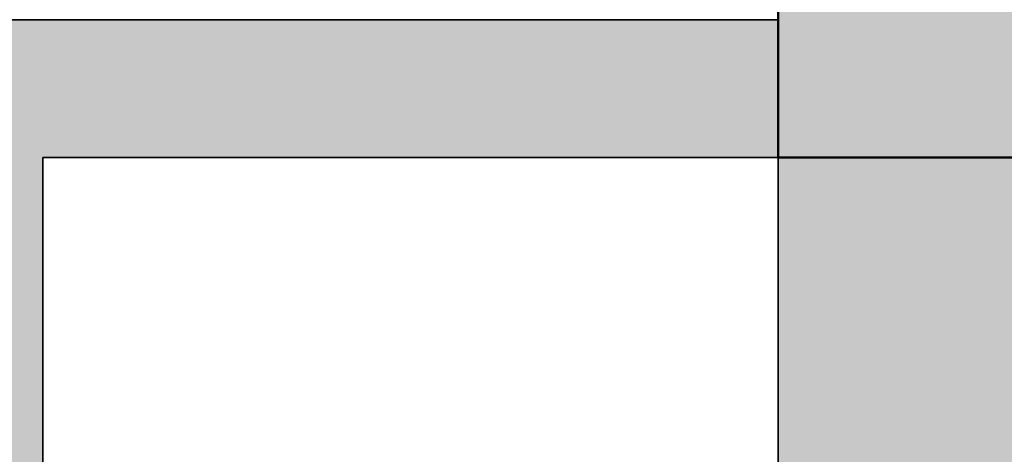
# Model space of a CAD drawing. Units: inches. Extents: x 1998 to 2588, y 1139 to 1977.
# Tile 59 of 134: x 2063 to 2095, y 1746 to 1760. Entities that reach past the tile are written whole.
import ezdxf

# ---------------------------------------------------------------- set-up
doc = ezdxf.new("R2010")
doc.units = ezdxf.units.IN
for name, color, linetype, lineweight in [('A-COLS-PATT', 250, 'Continuous', 13), ('A-WALL-PATT', 252, 'Continuous', 13), ('COLUMN', 10, 'Continuous', 50), ('WALL', 200, 'Continuous', 35)]:
    doc.layers.add(name, color=color, linetype=linetype, lineweight=lineweight)

msp = doc.modelspace()

# ---------------------------------------------------------------- hatches: boundary and pattern name
at = {"layer": 'A-COLS-PATT'}
h = msp.add_hatch(color=256, dxfattribs=at)
h.dxf.hatch_style = 1
h.paths.add_polyline_path([(2099.4125, 1888.7324), (2087.9729, 1888.7324), (2087.9729, 1868.3278), (2099.4125, 1868.3278)])
h.paths.add_polyline_path([(2234.4125, 1888.7324), (2222.9729, 1888.7324), (2222.9729, 1868.3278), (2234.4125, 1868.3278)])
h.paths.add_polyline_path([(2341.4729, 1886.637), (2330.0332, 1886.637), (2330.0332, 1866.2324), (2341.4729, 1866.2324)])
h.paths.add_polyline_path([(2507.8006, 1882.7324), (2487.396, 1882.7324), (2487.396, 1871.2927), (2507.8006, 1871.2927)])
h.paths.add_polyline_path([(2510.9729, 1766.672), (2490.5682, 1766.672), (2490.5682, 1755.2324), (2510.9729, 1755.2324)])
h.paths.add_polyline_path([(2345.9729, 1759.7324), (2334.5332, 1759.7324), (2334.5332, 1739.3278), (2345.9729, 1739.3278)])
h.paths.add_polyline_path([(2234.4125, 1774.3318), (2222.9729, 1774.3318), (2222.9729, 1753.9272), (2234.4125, 1753.9272)])
h.paths.add_polyline_path([(2099.4125, 1775.637), (2087.9729, 1775.637), (2087.9729, 1755.2324), (2099.4125, 1755.2324)])
h.paths.add_polyline_path([(2098.0956, 1593.7241), (2077.691, 1593.7241), (2077.691, 1582.2845), (2098.0956, 1582.2845)])
h.paths.add_polyline_path([(2227.4729, 1604.637), (2216.0332, 1604.637), (2216.0332, 1584.2324), (2227.4729, 1584.2324)])
h.paths.add_polyline_path([(2345.9729, 1647.5211), (2334.5332, 1647.5211), (2334.5332, 1627.1165), (2345.9729, 1627.1165)])
h.paths.add_polyline_path([(2522.3775, 1641.2324), (2501.9729, 1641.2324), (2501.9729, 1629.7927), (2522.3775, 1629.7927)])
h.paths.add_polyline_path([(2522.3775, 1480.7324), (2501.9729, 1480.7324), (2501.9729, 1469.2927), (2522.3775, 1469.2927)])
h.paths.add_polyline_path([(2345.9729, 1488.5616), (2334.5332, 1488.5616), (2334.5332, 1468.1569), (2345.9729, 1468.1569)])
h.paths.add_polyline_path([(2234.4125, 1486.137), (2227.4729, 1486.137), (2227.4729, 1465.7324), (2234.4125, 1465.7324)])
h.paths.add_polyline_path([(2227.4729, 1486.137), (2222.9729, 1486.137), (2222.9729, 1465.7324), (2227.4729, 1465.7324)])
h.paths.add_polyline_path([(2108.3775, 1470.2324), (2087.9729, 1470.2324), (2087.9729, 1458.7927), (2108.3775, 1458.7927)])
h.paths.add_polyline_path([(2096.9729, 1365.5012), (2087.9729, 1365.5012), (2087.9729, 1345.0966), (2096.9729, 1345.0966)])
h.paths.add_polyline_path([(2087.9729, 1365.5012), (2085.5332, 1365.5012), (2085.5332, 1345.0966), (2087.9729, 1345.0966)])
h.paths.add_polyline_path([(2234.4125, 1285.137), (2222.9729, 1285.137), (2222.9729, 1264.7324), (2234.4125, 1264.7324)])
h.paths.add_polyline_path([(2345.9729, 1285.137), (2334.5332, 1285.137), (2334.5332, 1264.7324), (2345.9729, 1264.7324)])
h.paths.add_polyline_path([(2503.1458, 1240.172), (2482.7412, 1240.172), (2482.7412, 1228.7324), (2503.1458, 1228.7324)])
h.paths.add_polyline_path([(2510.9729, 1369.172), (2490.5682, 1369.172), (2490.5682, 1357.7324), (2510.9729, 1357.7324)])
at = {"layer": 'A-WALL-PATT'}
h = msp.add_hatch(color=256, dxfattribs=at)
h.dxf.hatch_style = 1
h.paths.add_polyline_path([(2222.9729, 1888.7324), (2099.4125, 1888.7324), (2099.4125, 1879.7324), (2222.9729, 1879.7324)])
h.paths.add_polyline_path([(2096.9729, 1868.3278), (2087.9729, 1868.3278), (2087.9729, 1775.637), (2096.9729, 1775.637)])
h.paths.add_polyline_path([(2227.4729, 1868.3278), (2222.9729, 1868.3278), (2222.9729, 1774.3318), (2227.4729, 1774.3318)])
h.paths.add_polyline_path([(2188.3019, 1759.7324), (2138.6074, 1759.7324), (2099.4125, 1759.7324), (2099.4125, 1755.2324), (2176.9729, 1755.2324), (2188.3019, 1755.2324)])
h.paths.add_polyline_path([(2087.9729, 1759.7324), (2059.4729, 1759.7324), (2059.4729, 1702.7324), (2087.9729, 1702.7324), (2087.9729, 1707.2324), (2063.9729, 1707.2324), (2063.9729, 1755.2324), (2087.9729, 1755.2324)])
h.paths.add_polyline_path([(2096.9729, 1755.2324), (2087.9729, 1755.2324), (2087.9729, 1707.2324), (2096.9729, 1707.2324)])
h.paths.add_polyline_path([(2187.0461, 1707.2324), (2105.9729, 1707.2324), (2096.9729, 1707.2324), (2087.9729, 1707.2324), (2087.9729, 1702.7324), (2105.9729, 1702.7324), (2114.9729, 1702.7324), (2187.0461, 1702.7324)])
h.paths.add_polyline_path([(2181.4729, 1719.2028), (2176.9729, 1719.2028), (2176.9729, 1707.2324), (2181.4729, 1707.2324)])
h.paths.add_polyline_path([(2216.0332, 1588.7324), (2114.9729, 1588.7324), (2105.9729, 1588.7324), (2105.9729, 1584.2324), (2216.0332, 1584.2324)])
h.paths.add_polyline_path([(2077.691, 1588.7324), (2061.4729, 1588.7324), (2061.4729, 1584.2324), (2077.691, 1584.2324)])
h.paths.add_polyline_path([(2105.9729, 1588.7324), (2098.0956, 1588.7324), (2098.0956, 1584.2324), (2105.9729, 1584.2324)])
h.paths.add_polyline_path([(2114.9729, 1596.2642), (2110.1012, 1596.2642), (2105.9729, 1596.2642), (2105.9729, 1588.7324), (2114.9729, 1588.7324)])
h.paths.add_polyline_path([(2114.9729, 1584.2324), (2105.9729, 1584.2324), (2105.9729, 1580.249), (2110.1012, 1580.249), (2114.9729, 1580.249)])
h.paths.add_polyline_path([(2114.9729, 1547.7716), (2110.1012, 1547.7716, -0.0318759), (2105.9729, 1548.035), (2105.9729, 1470.2324), (2108.3775, 1470.2324), (2108.3775, 1465.7324), (2186.2943, 1465.7324), (2186.2943, 1470.2324), (2114.9729, 1470.2324)])
h.paths.add_polyline_path([(2227.4729, 1584.2324), (2222.9729, 1584.2324), (2222.9729, 1486.137), (2227.4729, 1486.137)])
h.paths.add_polyline_path([(2295.4138, 1593.2324), (2227.4729, 1593.2324), (2227.4729, 1588.7324), (2295.4138, 1588.7324), (2295.4138, 1591.8729)])
h.paths.add_polyline_path([(2345.9729, 1627.1165), (2341.4729, 1627.1165), (2341.4729, 1593.2324), (2337.2869, 1593.2324), (2337.2869, 1591.8729), (2337.2869, 1588.7324), (2345.9729, 1588.7324)])
h.paths.add_polyline_path([(2291.9729, 1588.7324), (2287.4729, 1588.7324), (2287.4729, 1522.7324), (2291.9729, 1522.7324)])
h.paths.add_polyline_path([(2291.9729, 1522.7324), (2287.4729, 1522.7324), (2227.4729, 1522.7324), (2227.4729, 1518.2324), (2291.9729, 1518.2324)])
h.paths.add_polyline_path([(2295.7347, 1519.5919), (2295.7347, 1522.7324), (2291.9729, 1522.7324), (2291.9729, 1518.2324), (2295.7347, 1518.2324)])
h.paths.add_polyline_path([(2345.9729, 1522.7324), (2337.6078, 1522.7324), (2337.6078, 1519.5919), (2337.6078, 1518.2324), (2341.4729, 1518.2324), (2341.4729, 1488.5616), (2345.9729, 1488.5616)])
h.paths.add_polyline_path([(2345.9729, 1468.1569), (2341.4729, 1468.1569), (2341.4729, 1374.2324), (2227.4729, 1374.2324), (2227.4729, 1369.7324), (2345.9729, 1369.7324)])
h.paths.add_polyline_path([(2345.9729, 1369.7324), (2341.4729, 1369.7324), (2341.4729, 1362.2324), (2345.9729, 1362.2324)])
h.paths.add_polyline_path([(2345.9729, 1317.7324), (2345.9729, 1322.2324), (2341.4729, 1322.2324), (2341.4729, 1285.137), (2345.9729, 1285.137)], flags=17)
h.paths.add_polyline_path([(2356.2096, 1322.2324), (2345.9729, 1322.2324), (2345.9729, 1317.7324), (2356.2096, 1317.7324), (2356.2096, 1319.3088)], flags=17)
h.paths.add_polyline_path([(2393.9729, 1322.2324), (2375.6999, 1322.2324), (2375.6999, 1319.3088, -0.0202458), (2375.636, 1317.7324), (2393.9729, 1317.7324)], flags=17)
h.paths.add_polyline_path([(2398.4729, 1322.2324), (2393.9729, 1322.2324), (2393.9729, 1317.7324), (2393.9729, 1237.7324), (2345.9729, 1237.7324), (2345.9729, 1264.7324), (2341.4729, 1264.7324), (2341.4729, 1228.7324), (2393.9729, 1228.7324), (2482.7412, 1228.7324), (2482.7412, 1237.7324), (2398.4729, 1237.7324), (2398.4729, 1297.1029)])
h.paths.add_polyline_path([(2398.4729, 1362.2324), (2393.9729, 1362.2324), (2393.9729, 1357.7324), (2398.4729, 1357.7324)])
h.paths.add_polyline_path([(2345.9729, 1329.7549), (2341.4729, 1329.7549), (2341.4729, 1322.2324), (2345.9729, 1322.2324)])

# ---------------------------------------------------------------- linework, layer by layer
at = {"layer": 'COLUMN'}
msp.add_lwpolyline([(2087.9729, 1775.637), (2099.4125, 1775.637), (2099.4125, 1755.2324), (2087.9729, 1755.2324)], close=True, dxfattribs=at)
at = {"layer": 'WALL'}
for p, q in [((2087.9729, 1888.7324), (2087.9729, 1755.2324)), ((2087.9729, 1759.7324), (2059.4729, 1759.7324)), ((2087.9729, 1755.2324), (2063.9729, 1755.2324)), ((2063.9729, 1755.2324), (2063.9729, 1707.2324)), ((2087.9729, 1755.2324), (2138.6074, 1755.2324)), ((2087.9729, 1755.2324), (2087.9729, 1702.7324))]:
    msp.add_line(p, q, dxfattribs=at)

doc.saveas('drawing.dxf')
